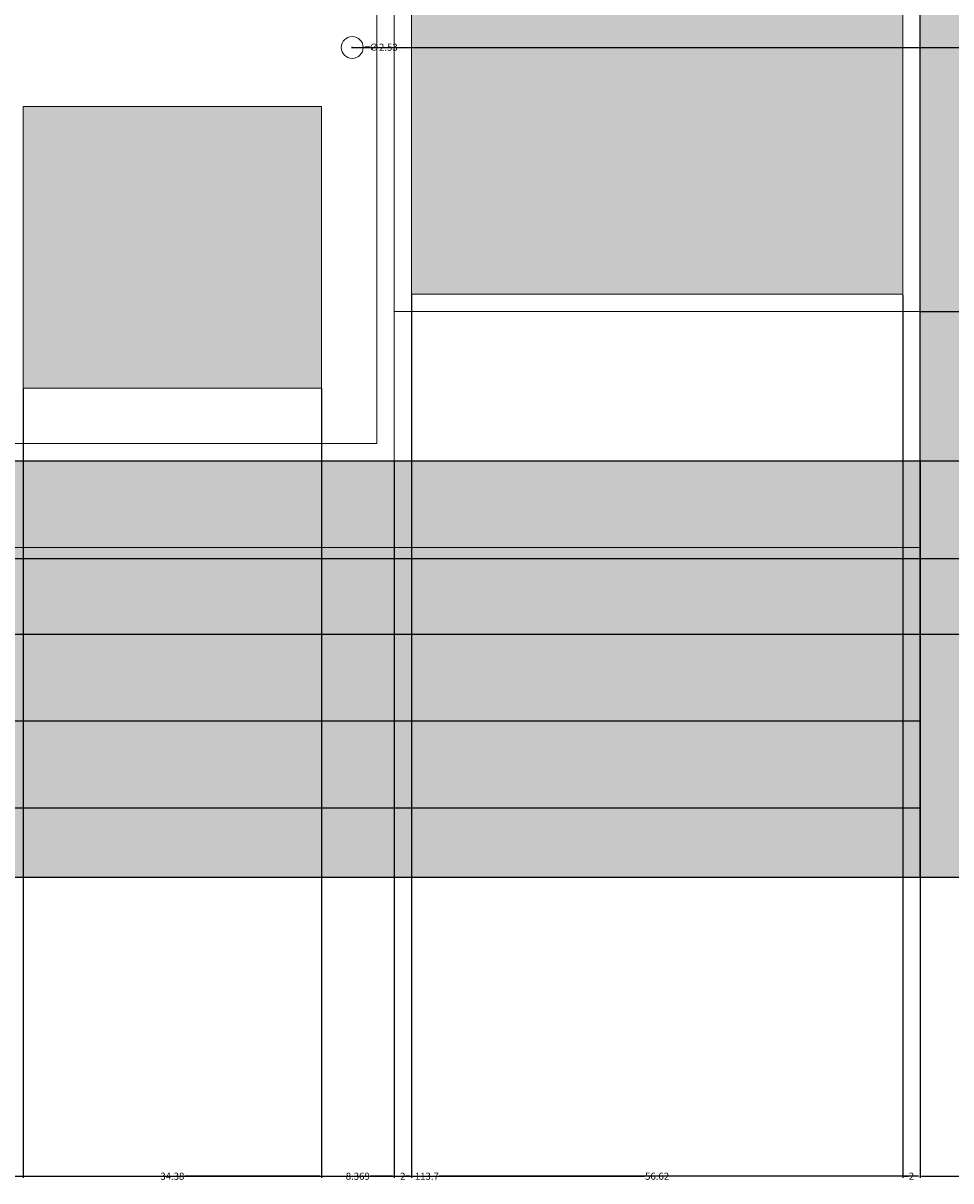
# Model space of a CAD drawing. Units: inches. Extents: x 36 to 594, y 79 to 831.
# Tile 2 of 30: x 114 to 221, y 79 to 213. Entities that reach past the tile are written whole.
import ezdxf

# ---------------------------------------------------------------- set-up
doc = ezdxf.new("R2010")
doc.units = ezdxf.units.IN
doc.header["$MEASUREMENT"] = 0
for name, color, linetype, lineweight in [('A-ANNO-DIMS', 2, 'Continuous', 18), ('A-DOOR', 3, 'Continuous', 18), ('A-ELEV', 7, 'Continuous', 25), ('A-ELEV-PATT', 8, 'Continuous', 13)]:
    doc.layers.add(name, color=color, linetype=linetype, lineweight=lineweight)
doc.styles.get("Standard").update_dxf_attribs({"font": 'arial.ttf'})
doc.dimstyles.get("Standard").update_dxf_attribs({"dimtxt": 0.8125, "dimasz": 0.18, "dimexe": 0.18, "dimexo": 0.0625, "dimgap": 0.09, "dimtad": 0, "dimtih": 1, "dimtoh": 1, "dimdec": 4, "dimzin": 0, "dimdsep": 46, "dimlunit": 4, "dimtxsty": 'Standard', "dimcen": 0.09, "dimadec": 0, "dimazin": 0, "dimtfac": 1, "dimtdec": 4, "dimtofl": 0, "dimtmove": 0, "dimatfit": 3, "dimfxl": 1, "dimtolj": 1, "dimtzin": 0, "dimarcsym": 0})

# ---------------------------------------------------------------- blocks, each defined once
blk = doc.blocks.new('*D8')
at = {"layer": 'A-ANNO-DIMS', "color": 0, "lineweight": -2, "transparency": 16777216}
for p, q in [((103.34, 114.15), (103.34, 79.53)), ((217.03, 114.15), (217.03, 79.53)), ((103.52, 79.71), (158.76, 79.71)), ((216.85, 79.71), (161.6, 79.71))]:
    blk.add_line(p, q, dxfattribs=at)
at = {"layer": 'A-ANNO-DIMS', "color": 0, "transparency": 16777216}
for points in [[(103.52, 79.74), (103.52, 79.68), (103.34, 79.71)], [(216.85, 79.74), (216.85, 79.68), (217.03, 79.71)]]:
    blk.add_solid(points, dxfattribs=at)
at = {"layer": 'Defpoints', "color": 0, "transparency": 16777216}
for p in [(103.34, 114.21), (217.03, 114.21), (217.03, 79.71)]:
    blk.add_point(p, dxfattribs=at)
at = {"layer": 'A-ANNO-DIMS', "color": 0, "transparency": 16777216, "insert": (160.18, 79.71), "char_height": 0.812, "attachment_point": 5}
blk.add_mtext('\\A1;113.7', dxfattribs=at)
blk = doc.blocks.new('*D9')
at = {"layer": 'A-ANNO-DIMS', "color": 0, "lineweight": -2, "transparency": 16777216}
for p, q in [((254.03, 142.15), (254.03, 79.53)), ((217.03, 114.15), (217.03, 79.53)), ((217.21, 79.71), (234.86, 79.71)), ((253.85, 79.71), (236.2, 79.71))]:
    blk.add_line(p, q, dxfattribs=at)
at = {"layer": 'A-ANNO-DIMS', "color": 0, "transparency": 16777216}
for points in [[(217.21, 79.74), (217.21, 79.68), (217.03, 79.71)], [(253.85, 79.74), (253.85, 79.68), (254.03, 79.71)]]:
    blk.add_solid(points, dxfattribs=at)
at = {"layer": 'Defpoints', "color": 0, "transparency": 16777216}
for p in [(254.03, 142.21), (217.03, 114.21), (254.03, 79.71)]:
    blk.add_point(p, dxfattribs=at)
at = {"layer": 'A-ANNO-DIMS', "color": 0, "transparency": 16777216, "insert": (235.53, 79.71), "char_height": 0.812, "attachment_point": 5}
blk.add_mtext('\\A1;37', dxfattribs=at)
blk = doc.blocks.new('*D28')
at = {"layer": 'A-ANNO-DIMS', "color": 0, "lineweight": -2, "transparency": 16777216}
for p, q in [((269.3, 796.05), (37.49, 796.05)), ((37.67, 795.87), (37.67, 455.63)), ((37.67, 114.39), (37.67, 454.62)), ((94.8, 114.21), (37.49, 114.21))]:
    blk.add_line(p, q, dxfattribs=at)
at = {"layer": 'A-ANNO-DIMS', "color": 0, "transparency": 16777216}
for points in [[(37.64, 795.87), (37.7, 795.87), (37.67, 796.05)], [(37.64, 114.39), (37.7, 114.39), (37.67, 114.21)]]:
    blk.add_solid(points, dxfattribs=at)
at = {"layer": 'Defpoints', "color": 0, "transparency": 16777216}
for p in [(37.67, 796.05), (269.36, 796.05), (94.87, 114.21)]:
    blk.add_point(p, dxfattribs=at)
at = {"layer": 'A-ANNO-DIMS', "color": 0, "transparency": 16777216, "insert": (37.67, 455.13), "char_height": 0.812, "attachment_point": 5}
blk.add_mtext('\\A1;681.8', dxfattribs=at)
blk = doc.blocks.new('*D63')
at = {"layer": 'A-ANNO-DIMS', "color": 0, "lineweight": -2, "transparency": 16777216}
for p, q in [((113.66, 170.54), (113.66, 79.53)), ((148.04, 170.54), (148.04, 79.53)), ((113.84, 79.71), (129.39, 79.71)), ((147.86, 79.71), (132.31, 79.71))]:
    blk.add_line(p, q, dxfattribs=at)
at = {"layer": 'A-ANNO-DIMS', "color": 0, "transparency": 16777216}
for points in [[(113.84, 79.74), (113.84, 79.68), (113.66, 79.71)], [(147.86, 79.74), (147.86, 79.68), (148.04, 79.71)]]:
    blk.add_solid(points, dxfattribs=at)
at = {"layer": 'Defpoints', "color": 0, "transparency": 16777216}
for p in [(113.66, 170.6), (148.04, 170.6), (148.04, 79.71)]:
    blk.add_point(p, dxfattribs=at)
at = {"layer": 'A-ANNO-DIMS', "color": 0, "transparency": 16777216, "insert": (130.85, 79.71), "char_height": 0.812, "attachment_point": 5}
blk.add_mtext('\\A1;34.38', dxfattribs=at)
blk = doc.blocks.new('*D64')
at = {"layer": 'A-ANNO-DIMS', "color": 0, "lineweight": -2, "transparency": 16777216}
for p, q in [((148.04, 170.54), (148.04, 79.53)), ((156.41, 162.15), (156.41, 79.53)), ((148.22, 79.71), (150.76, 79.71)), ((156.23, 79.71), (153.68, 79.71))]:
    blk.add_line(p, q, dxfattribs=at)
at = {"layer": 'A-ANNO-DIMS', "color": 0, "transparency": 16777216}
for points in [[(148.22, 79.74), (148.22, 79.68), (148.04, 79.71)], [(156.23, 79.74), (156.23, 79.68), (156.41, 79.71)]]:
    blk.add_solid(points, dxfattribs=at)
at = {"layer": 'Defpoints', "color": 0, "transparency": 16777216}
for p in [(148.04, 170.6), (156.41, 162.21), (156.41, 79.71)]:
    blk.add_point(p, dxfattribs=at)
at = {"layer": 'A-ANNO-DIMS', "color": 0, "transparency": 16777216, "insert": (152.22, 79.71), "char_height": 0.812, "attachment_point": 5}
blk.add_mtext('\\A1;8.369', dxfattribs=at)
blk = doc.blocks.new('*D65')
at = {"layer": 'A-ANNO-DIMS', "color": 0, "lineweight": -2, "transparency": 16777216}
for p, q in [((158.41, 181.36), (158.41, 79.53)), ((156.41, 162.15), (156.41, 79.53)), ((156.59, 79.71), (157.05, 79.71)), ((158.23, 79.71), (157.77, 79.71))]:
    blk.add_line(p, q, dxfattribs=at)
at = {"layer": 'A-ANNO-DIMS', "color": 0, "transparency": 16777216}
for points in [[(156.59, 79.74), (156.59, 79.68), (156.41, 79.71)], [(158.23, 79.74), (158.23, 79.68), (158.41, 79.71)]]:
    blk.add_solid(points, dxfattribs=at)
at = {"layer": 'Defpoints', "color": 0, "transparency": 16777216}
for p in [(158.41, 181.42), (156.41, 162.21), (158.41, 79.71)]:
    blk.add_point(p, dxfattribs=at)
at = {"layer": 'A-ANNO-DIMS', "color": 0, "transparency": 16777216, "insert": (157.41, 79.71), "char_height": 0.812, "attachment_point": 5}
blk.add_mtext('\\A1;2', dxfattribs=at)
blk = doc.blocks.new('*D66')
at = {"layer": 'A-ANNO-DIMS', "color": 0, "lineweight": -2, "transparency": 16777216}
for p, q in [((158.41, 181.36), (158.41, 79.53)), ((215.03, 181.36), (215.03, 79.53)), ((158.59, 79.71), (185.26, 79.71)), ((214.85, 79.71), (188.17, 79.71))]:
    blk.add_line(p, q, dxfattribs=at)
at = {"layer": 'A-ANNO-DIMS', "color": 0, "transparency": 16777216}
for points in [[(158.59, 79.74), (158.59, 79.68), (158.41, 79.71)], [(214.85, 79.74), (214.85, 79.68), (215.03, 79.71)]]:
    blk.add_solid(points, dxfattribs=at)
at = {"layer": 'Defpoints', "color": 0, "transparency": 16777216}
for p in [(158.41, 181.42), (215.03, 181.42), (215.03, 79.71)]:
    blk.add_point(p, dxfattribs=at)
at = {"layer": 'A-ANNO-DIMS', "color": 0, "transparency": 16777216, "insert": (186.72, 79.71), "char_height": 0.812, "attachment_point": 5}
blk.add_mtext('\\A1;56.62', dxfattribs=at)
blk = doc.blocks.new('*D67')
at = {"layer": 'A-ANNO-DIMS', "color": 0, "lineweight": -2, "transparency": 16777216}
for p, q in [((215.03, 181.36), (215.03, 79.53)), ((217.03, 162.15), (217.03, 79.53)), ((215.21, 79.71), (215.67, 79.71)), ((216.85, 79.71), (216.39, 79.71))]:
    blk.add_line(p, q, dxfattribs=at)
at = {"layer": 'A-ANNO-DIMS', "color": 0, "transparency": 16777216}
for points in [[(215.21, 79.74), (215.21, 79.68), (215.03, 79.71)], [(216.85, 79.74), (216.85, 79.68), (217.03, 79.71)]]:
    blk.add_solid(points, dxfattribs=at)
at = {"layer": 'Defpoints', "color": 0, "transparency": 16777216}
for p in [(215.03, 181.42), (217.03, 162.21), (217.03, 79.71)]:
    blk.add_point(p, dxfattribs=at)
at = {"layer": 'A-ANNO-DIMS', "color": 0, "transparency": 16777216, "insert": (216.03, 79.71), "char_height": 0.812, "attachment_point": 5}
blk.add_mtext('\\A1;2', dxfattribs=at)
blk = doc.blocks.new('*D74')
at = {"layer": 'A-ANNO-DIMS', "color": 0, "lineweight": -2, "transparency": 16777216}
for p, q in [((217.09, 179.42), (592.85, 179.42)), ((592.67, 179.24), (592.67, 171.32)), ((592.67, 162.39), (592.67, 170.31)), ((217.09, 162.21), (592.85, 162.21))]:
    blk.add_line(p, q, dxfattribs=at)
at = {"layer": 'A-ANNO-DIMS', "color": 0, "transparency": 16777216}
for points in [[(592.64, 179.24), (592.7, 179.24), (592.67, 179.42)], [(592.64, 162.39), (592.7, 162.39), (592.67, 162.21)]]:
    blk.add_solid(points, dxfattribs=at)
at = {"layer": 'Defpoints', "color": 0, "transparency": 16777216}
for p in [(217.03, 179.42), (592.67, 179.42), (217.03, 162.21)]:
    blk.add_point(p, dxfattribs=at)
at = {"layer": 'A-ANNO-DIMS', "color": 0, "transparency": 16777216, "insert": (592.67, 170.82), "char_height": 0.812, "attachment_point": 5}
blk.add_mtext('\\A1;17.207', dxfattribs=at)
blk = doc.blocks.new('*D75')
at = {"layer": 'A-ANNO-DIMS', "color": 0, "lineweight": -2, "transparency": 16777216}
for p, q in [((215.09, 262.62), (592.85, 262.62)), ((592.67, 262.44), (592.67, 221.53)), ((592.67, 179.6), (592.67, 220.52)), ((217.09, 179.42), (592.85, 179.42))]:
    blk.add_line(p, q, dxfattribs=at)
at = {"layer": 'A-ANNO-DIMS', "color": 0, "transparency": 16777216}
for points in [[(592.64, 262.44), (592.7, 262.44), (592.67, 262.62)], [(592.64, 179.6), (592.7, 179.6), (592.67, 179.42)]]:
    blk.add_solid(points, dxfattribs=at)
at = {"layer": 'Defpoints', "color": 0, "transparency": 16777216}
for p in [(215.03, 262.62), (592.67, 262.62), (217.03, 179.42)]:
    blk.add_point(p, dxfattribs=at)
at = {"layer": 'A-ANNO-DIMS', "color": 0, "transparency": 16777216, "insert": (592.67, 221.02), "char_height": 0.812, "attachment_point": 5}
blk.add_mtext('\\A1;83.2', dxfattribs=at)
blk = doc.blocks.new('*D77')
at = {"layer": 'A-ANNO-DIMS', "color": 0, "lineweight": -2, "transparency": 16777216}
for p, q in [((151.64, 209.88), (592.85, 209.88)), ((592.67, 209.7), (592.67, 186.55)), ((592.67, 162.39), (592.67, 185.54)), ((156.47, 162.21), (592.85, 162.21))]:
    blk.add_line(p, q, dxfattribs=at)
at = {"layer": 'A-ANNO-DIMS', "color": 0, "transparency": 16777216}
for points in [[(592.64, 209.7), (592.7, 209.7), (592.67, 209.88)], [(592.64, 162.39), (592.7, 162.39), (592.67, 162.21)]]:
    blk.add_solid(points, dxfattribs=at)
at = {"layer": 'Defpoints', "color": 0, "transparency": 16777216}
for p in [(151.58, 209.88), (156.41, 162.21), (592.67, 162.21)]:
    blk.add_point(p, dxfattribs=at)
at = {"layer": 'A-ANNO-DIMS', "color": 0, "transparency": 16777216, "insert": (592.67, 186.05), "char_height": 0.812, "attachment_point": 5}
blk.add_mtext('\\A1;47.67', dxfattribs=at)
blk = doc.blocks.new('*D90')
at = {"layer": 'A-ANNO-DIMS', "color": 0, "lineweight": -2, "transparency": 16777216}
for p, q in [((255.97, 269.61), (37.49, 269.61)), ((37.67, 269.43), (37.67, 210.78)), ((37.67, 151.11), (37.67, 209.77)), ((253.97, 150.93), (37.49, 150.93))]:
    blk.add_line(p, q, dxfattribs=at)
at = {"layer": 'A-ANNO-DIMS', "color": 0, "transparency": 16777216}
for points in [[(37.64, 269.43), (37.7, 269.43), (37.67, 269.61)], [(37.64, 151.11), (37.7, 151.11), (37.67, 150.93)]]:
    blk.add_solid(points, dxfattribs=at)
at = {"layer": 'Defpoints', "color": 0, "transparency": 16777216}
for p in [(37.67, 269.61), (256.03, 269.61), (254.03, 150.93)]:
    blk.add_point(p, dxfattribs=at)
at = {"layer": 'A-ANNO-DIMS', "color": 0, "transparency": 16777216, "insert": (37.67, 210.27), "char_height": 0.812, "attachment_point": 5}
blk.add_mtext('\\A1;118.67', dxfattribs=at)
blk = doc.blocks.new('*D131')
at = {"layer": 'A-ANNO-DIMS', "color": 0, "lineweight": -2, "transparency": 16777216}
for p, q in [((151.49, 209.88), (151.67, 209.88)), ((151.58, 209.79), (151.58, 209.97)), ((153.61, 209.91), (153.03, 209.9))]:
    blk.add_line(p, q, dxfattribs=at)
at = {"layer": 'A-ANNO-DIMS', "color": 0, "transparency": 16777216}
blk.add_solid([(153.03, 209.93), (153.03, 209.87), (152.85, 209.9)], dxfattribs=at)
at = {"layer": 'Defpoints', "color": 0, "transparency": 16777216}
for p in [(150.31, 209.86), (152.85, 209.9)]:
    blk.add_point(p, dxfattribs=at)
at = {"layer": 'A-ANNO-DIMS', "color": 0, "transparency": 16777216, "insert": (155.19, 209.91), "char_height": 0.812, "attachment_point": 5}
blk.add_mtext('\\A1;∅2.53', dxfattribs=at)

msp = doc.modelspace()

# ---------------------------------------------------------------- hatches: boundary and pattern name
at = {"layer": 'A-ELEV-PATT'}
h = msp.add_hatch(color=256, dxfattribs=at)
h.dxf.hatch_style = 1
h.paths.add_polyline_path([(398.0873, 796.0465), (269.3592, 796.0465), (269.3592, 770.1455), (397.8159, 770.1455)])
h.paths.add_polyline_path([(397.7518, 764.0341), (269.3592, 764.0341), (269.3592, 630.0394), (341.8367, 630.0394), (341.8367, 720.595), (335.0881, 728.3699), (329.982, 735.3373), (345.3661, 727.7743), (397.1052, 702.3389)])
h.paths.add_polyline_path([(341.8367, 594.2124), (201.4189, 594.2124), (201.4189, 475.4136), (232.8216, 475.4136), (232.8216, 524.6037), (341.8367, 524.6037)])
h.paths.add_polyline_path([(177.525, 594.2124), (118.7598, 594.2124), (118.7598, 450.2124), (177.525, 450.2124)])
h.paths.add_polyline_path([(424.4958, 594.2124), (365.7306, 594.2124), (365.7306, 450.2124), (424.4958, 450.2124)])
h.paths.add_polyline_path([(241.3553, 404.2737), (355.8569, 404.2737), (355.8569, 355.0836), (424.5492, 355.0836), (424.5492, 425.7333), (118.7598, 426.2844), (118.7598, 355.0836), (241.3553, 355.0836)])
h.paths.add_polyline_path([(448.3898, 306.2124), (217.0273, 306.2124), (217.0273, 142.2124), (254.0293, 142.2124), (254.0293, 150.9347), (254.0293, 286.1802), (401.5491, 286.1802), (401.5491, 150.9347), (401.5491, 142.2124), (448.3898, 142.2124)])
h.paths.add_polyline_path([(448.3898, 142.2124), (401.5491, 142.2124), (217.0273, 142.2124), (217.0273, 114.2124), (448.3898, 114.2124)])
h.paths.add_polyline_path([(217.0273, 306.2124), (174.7353, 306.2124), (94.8658, 306.2124), (94.8658, 162.2124), (103.3368, 162.2124), (103.3368, 264.6224), (103.3368, 286.1802), (217.0273, 286.1802)])
h = msp.add_hatch(color=256, dxfattribs=at)
h.dxf.hatch_style = 1
h.set_gradient(color1=(0, 255, 255), color2=(16, 86, 137))
h.paths.add_polyline_path([(341.8367, 524.6037), (260.5056, 524.6037), (260.5056, 513.1224), (341.8367, 513.1224)])
h.paths.add_polyline_path([(341.8367, 511.1224), (260.5056, 511.1224), (260.5056, 475.4136), (341.8367, 475.4136)])
h.paths.add_polyline_path([(258.5056, 524.6037), (232.8216, 524.6037), (232.8216, 513.1224), (258.5056, 513.1224)])
h.paths.add_polyline_path([(355.8569, 404.2737), (269.0393, 404.2737), (269.0393, 392.7924), (355.8569, 392.7924)])
h.paths.add_polyline_path([(267.0393, 404.2737), (241.3553, 404.2737), (241.3553, 392.7924), (267.0393, 392.7924)])
h.paths.add_polyline_path([(355.8569, 390.7924), (269.0393, 390.7924), (269.0393, 355.0836), (355.8569, 355.0836)])
h.paths.add_polyline_path([(399.5491, 284.1802), (256.0293, 284.1802), (256.0293, 271.378), (399.5491, 271.378)])
h.paths.add_polyline_path([(317.3533, 259.1243), (262.3169, 259.1243), (262.3169, 200.6645), (317.3533, 200.6645)])
h.paths.add_polyline_path([(390.386, 259.1243), (335.3496, 259.1243), (335.3496, 200.6645), (390.386, 200.6645)])
h.paths.add_polyline_path([(390.386, 190.7697), (335.3496, 190.7697), (335.3496, 162.9881), (390.386, 162.9881)])
h.paths.add_polyline_path([(317.3533, 190.7697), (262.3169, 190.7697), (262.3169, 162.9881), (317.3533, 162.9881)])
h.paths.add_polyline_path([(215.0273, 262.6224), (158.4069, 262.6224), (158.4069, 181.4195), (215.0273, 181.4195)])
h.paths.add_polyline_path([(215.0273, 284.1802), (105.3368, 284.1802), (105.3368, 266.6224), (215.0273, 266.6224)])
h = msp.add_hatch(dxfattribs=at)
h.set_pattern_fill('ANSI33', color=256, scale=6.3, angle=135)
h.paths.add_polyline_path([(255.3555, 505.4499), (236.2911, 505.4499), (236.2911, 488.4928), (255.3555, 488.4928)])
h.paths.add_polyline_path([(255.3555, 484.4187), (236.2911, 484.4187), (236.2911, 475.4136), (255.3555, 475.4136)])
h.paths.add_polyline_path([(263.8892, 385.1199), (244.8248, 385.1199), (244.8248, 368.1628), (263.8892, 368.1628)])
h.paths.add_polyline_path([(263.8892, 364.0887), (244.8248, 364.0887), (244.8248, 355.0836), (263.8892, 355.0836)])
h.paths.add_polyline_path([(148.0383, 248.8663), (113.6593, 248.8663), (113.6593, 214.2237), (148.0383, 214.2237)])
h.paths.add_polyline_path([(148.0383, 203.057), (113.6593, 203.057), (113.6593, 170.5978), (148.0383, 170.5978)])
h = msp.add_hatch(color=256, dxfattribs=at)
h.dxf.hatch_style = 1
h.set_gradient(color1=(192, 192, 192), color2=(0, 0, 0))
h.paths.add_polyline_path([(243.19, 469.3251), (222.9132, 469.3251), (222.9132, 454.5571), (243.1634, 454.5571)])
h.paths.add_polyline_path([(264.4667, 469.2868), (244.1899, 469.2868), (244.1899, 454.5188), (264.4401, 454.5188)])
h.paths.add_polyline_path([(285.7435, 469.2484), (265.4667, 469.2484), (265.4667, 454.4804), (285.7168, 454.4804)])
h.paths.add_polyline_path([(307.0202, 469.2101), (286.7434, 469.2101), (286.7434, 454.4421), (306.9936, 454.4421)])
h.paths.add_polyline_path([(328.2969, 469.1717), (308.0201, 469.1717), (308.0201, 454.4037), (328.2703, 454.4037)])
h.paths.add_polyline_path([(341.8367, 469.1334), (329.2969, 469.1334), (329.2969, 454.3654), (341.8367, 454.3654)])
h.paths.add_polyline_path([(221.9133, 469.3635), (201.6365, 469.3635), (201.6365, 454.5955), (221.8866, 454.5955)])
h.paths.add_polyline_path([(145.3401, 349.1868), (125.0633, 349.1868), (125.0633, 334.4189), (145.3134, 334.4189)])
h.paths.add_polyline_path([(166.6168, 349.1485), (146.34, 349.1485), (146.34, 334.3805), (166.5902, 334.3805)])
h.paths.add_polyline_path([(187.8935, 349.1101), (167.6167, 349.1101), (167.6167, 334.3422), (187.8669, 334.3422)])
h.paths.add_polyline_path([(209.1703, 349.0718), (188.8935, 349.0718), (188.8935, 334.3038), (209.1436, 334.3038)])
h.paths.add_polyline_path([(230.447, 349.0335), (210.1702, 349.0335), (210.1702, 334.2655), (230.4204, 334.2655)])
h.paths.add_polyline_path([(251.7237, 348.9951), (231.4469, 348.9951), (231.4469, 334.2271), (251.6971, 334.2271)])
h.paths.add_polyline_path([(273.0005, 348.9568), (252.7236, 348.9568), (252.7236, 334.1888), (272.9738, 334.1888)])
h.paths.add_polyline_path([(294.2772, 348.9184), (274.0004, 348.9184), (274.0004, 334.1504), (294.2506, 334.1504)])
h.paths.add_polyline_path([(315.5539, 348.8801), (295.2771, 348.8801), (295.2771, 334.1121), (315.5273, 334.1121)])
h.paths.add_polyline_path([(336.8306, 348.8417), (316.5538, 348.8417), (316.5538, 334.0737), (336.804, 334.0737)])
h.paths.add_polyline_path([(358.1074, 348.8034), (337.8306, 348.8034), (337.8306, 334.0354), (358.0808, 334.0354)])
h.paths.add_polyline_path([(379.3841, 348.765), (359.1073, 348.765), (359.1073, 333.997), (379.3575, 333.997)])
h.paths.add_polyline_path([(400.6608, 348.7267), (380.384, 348.7267), (380.384, 333.9587), (400.6342, 333.9587)])
h.paths.add_polyline_path([(421.9376, 348.6883), (401.6608, 348.6883), (401.6608, 333.9204), (421.911, 333.9204)])
h.paths.add_polyline_path([(103.3368, 162.2124), (94.8658, 162.2124), (94.8658, 150.2124), (94.8658, 114.2124), (103.3368, 114.2124)])
h.paths.add_polyline_path([(217.0273, 132.2124), (103.3368, 132.2124), (103.3368, 122.2124), (217.0273, 122.2124)])
h.paths.add_polyline_path([(217.0273, 122.2124), (103.3368, 122.2124), (103.3368, 114.2124), (217.0273, 114.2124)])
h.paths.add_polyline_path([(217.0273, 142.2124), (174.7353, 142.2124), (103.3368, 142.2124), (103.3368, 132.2124), (217.0273, 132.2124)])
h.paths.add_polyline_path([(217.0273, 152.2124), (103.3368, 152.2124), (103.3368, 142.2124), (174.7353, 142.2124), (217.0273, 142.2124)])
h.paths.add_polyline_path([(217.0273, 162.2124), (103.3368, 162.2124), (103.3368, 152.2124), (217.0273, 152.2124)])

# ---------------------------------------------------------------- linework, layer by layer
at = {"layer": 'A-DOOR'}
msp.add_line((103.3368, 152.2124), (217.0273, 152.2124), dxfattribs=at)
for points in [[(103.3368, 162.2124), (156.4069, 162.2124), (156.4069, 264.6224), (103.3368, 264.6224)], [(156.4069, 264.6224), (217.0273, 264.6224), (217.0273, 179.4195), (156.4069, 179.4195)], [(105.3368, 164.2124), (154.4069, 164.2124), (154.4069, 262.6224), (105.3368, 262.6224)], [(158.4069, 262.6224), (215.0273, 262.6224), (215.0273, 181.4195), (158.4069, 181.4195)], [(113.6593, 203.057), (148.0383, 203.057), (148.0383, 170.5978), (113.6593, 170.5978)]]:
    msp.add_lwpolyline(points, close=True, dxfattribs=at)
msp.add_circle((151.5799, 209.8823), 1.2674, dxfattribs=at)
at = {"layer": 'A-ELEV'}
for p, q in [((217.0273, 114.2124), (217.0273, 306.2124)), ((94.8658, 162.2124), (217.0273, 162.2124)), ((103.3368, 142.2124), (174.7353, 142.2124)), ((174.7353, 142.2124), (448.3898, 142.2124)), ((103.3368, 132.2124), (217.0273, 132.2124)), ((103.3368, 122.2124), (217.0273, 122.2124)), ((84.3711, 114.2124), (558.1689, 114.2124))]:
    msp.add_line(p, q, dxfattribs=at)

# ---------------------------------------------------------------- dimensions: what is measured, and where the dimension line sits
at = {"layer": 'A-ANNO-DIMS'}
for base, p1, p2, override, picture, middle in [((37.6733, 796.0465), (94.8658, 114.2124), (269.3592, 796.0465), {"dimdec": 1, "dimlfac": 1, "dimrnd": 0, "dimzin": 0, "dimdsep": 46, "dimlunit": 2}, '*D28', (37.6733, 455.1294)), ((37.6733, 269.6084), (254.0293, 150.9347), (256.0293, 269.6084), {"dimdec": 2, "dimlfac": 1, "dimrnd": 0, "dimzin": 0, "dimdsep": 46, "dimlunit": 2}, '*D90', (37.6733, 210.2716)), ((592.6689, 262.6224), (217.0273, 179.4195), (215.0273, 262.6224), {"dimdec": 1, "dimlfac": 1, "dimrnd": 0, "dimzin": 0, "dimdsep": 46, "dimlunit": 2}, '*D75', (592.6689, 221.021)), ((592.6689, 162.2124), (151.5799, 209.8823), (156.4069, 162.2124), {"dimdec": 2, "dimlfac": 1, "dimrnd": 0, "dimzin": 0, "dimdsep": 46, "dimlunit": 2}, '*D77', (592.6689, 186.0473)), ((592.6689, 179.4195), (217.0273, 162.2124), (217.0273, 179.4195), {"dimdec": 3, "dimlfac": 1, "dimrnd": 0, "dimzin": 0, "dimdsep": 46, "dimlunit": 2}, '*D74', (592.6689, 170.8159))]:
    dim = msp.add_linear_dim(base=base, p1=p1, p2=p2, angle=90, dimstyle='Standard', override=override, dxfattribs=at)
    dim.commit()
    dim.dimension.update_dxf_attribs({"geometry": picture, "text_midpoint": middle})
dim = msp.add_diameter_dim_2p(p1=(150.3127, 209.8639), p2=(152.8472, 209.9007), dimstyle='Standard', override={"dimdec": 2, "dimlfac": 1, "dimrnd": 0, "dimzin": 0, "dimdsep": 46, "dimlunit": 2}, dxfattribs=at)
dim.commit()
dim.dimension.update_dxf_attribs({"geometry": '*D131', "text_midpoint": (153.6075, 209.9117), "dimtype": 163})
for base, p1, p2, override, picture, middle in [((158.4069, 79.7124), (156.4069, 162.2124), (158.4069, 181.4195), {"dimdec": 0, "dimlfac": 1, "dimrnd": 0, "dimzin": 0, "dimdsep": 46, "dimlunit": 2}, '*D65', (157.4069, 79.7124)), ((215.0273, 79.7124), (158.4069, 181.4195), (215.0273, 181.4195), {"dimdec": 2, "dimlfac": 1, "dimrnd": 0, "dimzin": 0, "dimdsep": 46, "dimlunit": 2}, '*D66', (186.7171, 79.7124)), ((217.0273, 79.7124), (215.0273, 181.4195), (217.0273, 162.2124), {"dimdec": 0, "dimlfac": 1, "dimrnd": 0, "dimzin": 0, "dimdsep": 46, "dimlunit": 2}, '*D67', (216.0273, 79.7124)), ((148.0383, 79.7124), (113.6593, 170.5978), (148.0383, 170.5978), {"dimdec": 2, "dimlfac": 1, "dimrnd": 0, "dimzin": 0, "dimdsep": 46, "dimlunit": 2}, '*D63', (130.8488, 79.7124)), ((156.4069, 79.7124), (148.0383, 170.5978), (156.4069, 162.2124), {"dimdec": 3, "dimlfac": 1, "dimrnd": 0, "dimzin": 0, "dimdsep": 46, "dimlunit": 2}, '*D64', (152.2226, 79.7124)), ((254.0293, 79.7124), (217.0273, 114.2124), (254.0293, 142.2124), {"dimdec": 0, "dimlfac": 1, "dimrnd": 0, "dimzin": 0, "dimdsep": 46, "dimlunit": 2}, '*D9', (235.5283, 79.7124)), ((217.0273, 79.7124), (103.3368, 114.2124), (217.0273, 114.2124), {"dimdec": 1, "dimlfac": 1, "dimrnd": 0, "dimzin": 0, "dimdsep": 46, "dimlunit": 2}, '*D8', (160.182, 79.7124))]:
    dim = msp.add_linear_dim(base=base, p1=p1, p2=p2, dimstyle='Standard', override=override, dxfattribs=at)
    dim.commit()
    dim.dimension.update_dxf_attribs({"geometry": picture, "text_midpoint": middle})

doc.saveas('drawing.dxf')
